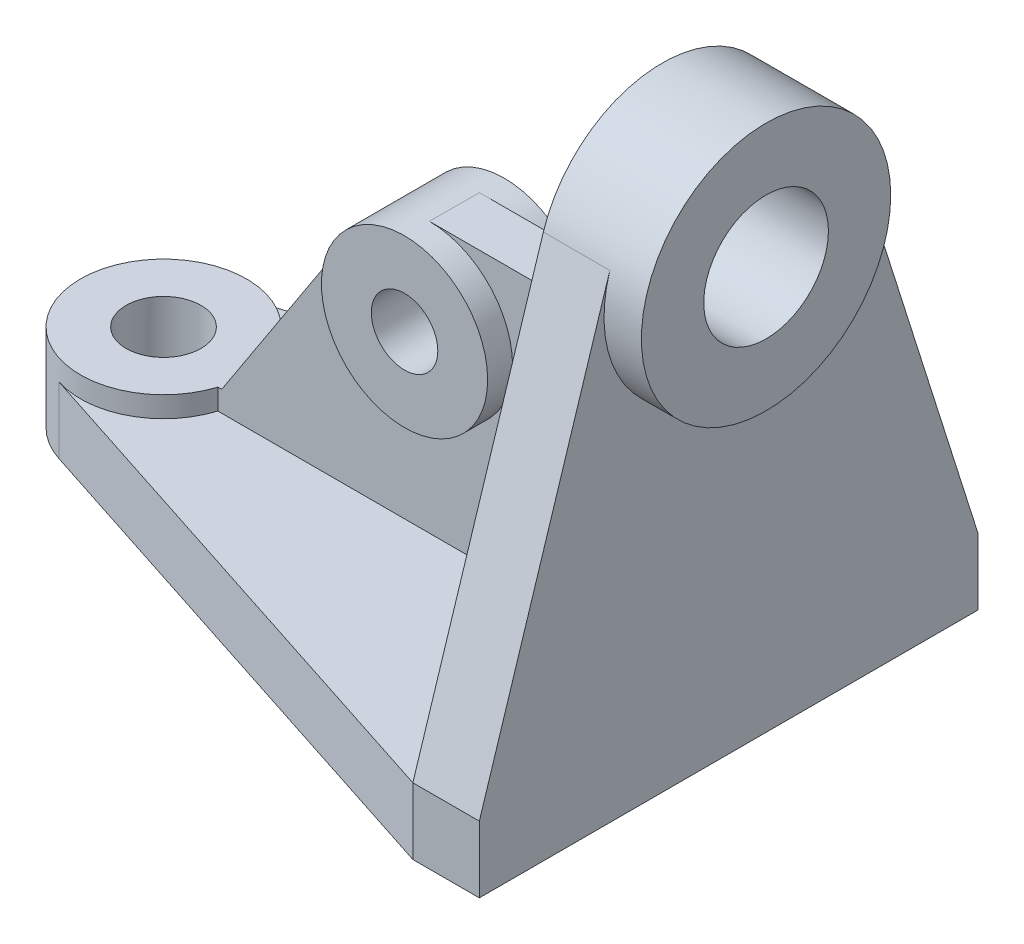
ISO-10303-21;
HEADER;
FILE_DESCRIPTION(('STEP AP214'),'2;1');
FILE_NAME('part.step','',(''),(''),'','','');
FILE_SCHEMA(('AUTOMOTIVE_DESIGN { 1 0 10303 214 1 1 1 1 }'));
ENDSEC;
DATA;
#1=APPLICATION_CONTEXT('core data for automotive mechanical design processes');
#2=APPLICATION_PROTOCOL_DEFINITION('international standard','automotive_design',2000,#1);
#3=PRODUCT_CONTEXT('',#1,'mechanical');
#4=PRODUCT('Part','Part','',(#3));
#5=PRODUCT_RELATED_PRODUCT_CATEGORY('part','',(#4));
#6=PRODUCT_DEFINITION_FORMATION('','',#4);
#7=PRODUCT_DEFINITION_CONTEXT('part definition',#1,'design');
#8=PRODUCT_DEFINITION('design','',#6,#7);
#9=PRODUCT_DEFINITION_SHAPE('','',#8);
#10=(LENGTH_UNIT() NAMED_UNIT(*) SI_UNIT(.MILLI.,.METRE.));
#11=(NAMED_UNIT(*) PLANE_ANGLE_UNIT() SI_UNIT($,.RADIAN.));
#12=(NAMED_UNIT(*) SI_UNIT($,.STERADIAN.) SOLID_ANGLE_UNIT());
#13=UNCERTAINTY_MEASURE_WITH_UNIT(LENGTH_MEASURE(1.E-05),#10,'distance_accuracy_value','');
#14=(GEOMETRIC_REPRESENTATION_CONTEXT(3) GLOBAL_UNCERTAINTY_ASSIGNED_CONTEXT((#13)) GLOBAL_UNIT_ASSIGNED_CONTEXT((#10,
#11,#12)) REPRESENTATION_CONTEXT('',''));
#15=CARTESIAN_POINT('',(0.,0.,0.));
#16=DIRECTION('',(0.,0.,1.));
#17=DIRECTION('',(1.,0.,0.));
#18=AXIS2_PLACEMENT_3D('',#15,#16,#17);
#19=CARTESIAN_POINT('',(-136.,-90.,0.));
#20=DIRECTION('',(0.,-1.,0.));
#21=DIRECTION('',(0.,0.,-1.));
#22=AXIS2_PLACEMENT_3D('',#19,#20,#21);
#23=PLANE('',#22);
#24=CARTESIAN_POINT('',(-136.,-90.,0.));
#25=DIRECTION('',(0.,1.,0.));
#26=DIRECTION('',(0.,0.,1.));
#27=AXIS2_PLACEMENT_3D('',#24,#25,#26);
#28=CIRCLE('',#27,20.);
#29=CARTESIAN_POINT('',(-116.921215971661,-90.,-5.99999999999999));
#30=VERTEX_POINT('',#29);
#31=CARTESIAN_POINT('',(-142.177666107614,-90.,-19.0219988818955));
#32=VERTEX_POINT('',#31);
#33=EDGE_CURVE('E216',#30,#32,#28,.T.);
#34=ORIENTED_EDGE('',*,*,#33,.F.);
#35=DIRECTION('',(1.,0.,0.));
#36=VECTOR('',#35,1.);
#37=CARTESIAN_POINT('',(-16.,-90.,-6.));
#38=LINE('',#37,#36);
#39=CARTESIAN_POINT('',(-16.,-90.,-6.));
#40=VERTEX_POINT('',#39);
#41=EDGE_CURVE('E53',#30,#40,#38,.T.);
#42=ORIENTED_EDGE('',*,*,#41,.T.);
#43=DIRECTION('',(0.,0.,-1.));
#44=VECTOR('',#43,1.);
#45=CARTESIAN_POINT('',(-16.,-90.,60.));
#46=LINE('',#45,#44);
#47=CARTESIAN_POINT('',(-16.,-90.,-60.));
#48=VERTEX_POINT('',#47);
#49=EDGE_CURVE('E276',#40,#48,#46,.T.);
#50=ORIENTED_EDGE('',*,*,#49,.T.);
#51=DIRECTION('',(0.951099944094773,0.,-0.30888330538072));
#52=VECTOR('',#51,1.);
#53=CARTESIAN_POINT('',(-16.,-90.,-60.));
#54=LINE('',#53,#52);
#55=EDGE_CURVE('E230',#32,#48,#54,.T.);
#56=ORIENTED_EDGE('',*,*,#55,.F.);
#57=EDGE_LOOP('',(#34,#42,#50,#56));
#58=FACE_BOUND('',#57,.T.);
#59=ADVANCED_FACE('F39',(#58),#23,.F.);
#60=DIRECTION('',(1.,0.,0.));
#61=VECTOR('',#60,1.);
#62=CARTESIAN_POINT('',(-16.,-90.,6.));
#63=LINE('',#62,#61);
#64=CARTESIAN_POINT('',(-116.921215971661,-90.,5.99999999999999));
#65=VERTEX_POINT('',#64);
#66=CARTESIAN_POINT('',(-16.,-90.,6.));
#67=VERTEX_POINT('',#66);
#68=EDGE_CURVE('E65',#65,#67,#63,.T.);
#69=ORIENTED_EDGE('',*,*,#68,.F.);
#70=CARTESIAN_POINT('',(-142.177666107614,-90.,19.0219988818955));
#71=VERTEX_POINT('',#70);
#72=EDGE_CURVE('E218',#71,#65,#28,.T.);
#73=ORIENTED_EDGE('',*,*,#72,.F.);
#74=DIRECTION('',(-0.951099944094773,0.,-0.30888330538072));
#75=VECTOR('',#74,1.);
#76=CARTESIAN_POINT('',(-142.177666107614,-90.,19.0219988818955));
#77=LINE('',#76,#75);
#78=CARTESIAN_POINT('',(-16.,-90.,60.));
#79=VERTEX_POINT('',#78);
#80=EDGE_CURVE('E224',#79,#71,#77,.T.);
#81=ORIENTED_EDGE('',*,*,#80,.F.);
#82=EDGE_CURVE('E278',#79,#67,#46,.T.);
#83=ORIENTED_EDGE('',*,*,#82,.T.);
#84=EDGE_LOOP('',(#69,#73,#81,#83));
#85=FACE_BOUND('',#84,.T.);
#86=ADVANCED_FACE('F370',(#85),#23,.F.);
#87=CARTESIAN_POINT('',(-16.,-90.,-60.));
#88=DIRECTION('',(0.,0.302169479251962,-0.953254218877943));
#89=DIRECTION('',(0.,0.953254218877943,0.302169479251962));
#90=AXIS2_PLACEMENT_3D('',#87,#88,#89);
#91=PLANE('',#90);
#92=DIRECTION('',(0.,0.953254218877943,0.302169479251962));
#93=VECTOR('',#92,1.);
#94=CARTESIAN_POINT('',(0.,-90.,-60.));
#95=LINE('',#94,#93);
#96=CARTESIAN_POINT('',(0.,-90.,-60.));
#97=VERTEX_POINT('',#96);
#98=CARTESIAN_POINT('',(0.,9.06508437755886,-28.5976265663383));
#99=VERTEX_POINT('',#98);
#100=EDGE_CURVE('E269',#97,#99,#95,.T.);
#101=ORIENTED_EDGE('',*,*,#100,.F.);
#102=DIRECTION('',(1.,0.,0.));
#103=VECTOR('',#102,1.);
#104=CARTESIAN_POINT('',(-16.,-90.,-60.));
#105=LINE('',#104,#103);
#106=EDGE_CURVE('E270',#48,#97,#105,.T.);
#107=ORIENTED_EDGE('',*,*,#106,.F.);
#108=DIRECTION('',(0.,0.953254218877943,0.302169479251962));
#109=VECTOR('',#108,1.);
#110=CARTESIAN_POINT('',(-16.,-90.,-60.));
#111=LINE('',#110,#109);
#112=CARTESIAN_POINT('',(-16.,9.06508437755887,-28.5976265663383));
#113=VERTEX_POINT('',#112);
#114=EDGE_CURVE('E271',#48,#113,#111,.T.);
#115=ORIENTED_EDGE('',*,*,#114,.T.);
#116=DIRECTION('',(1.,0.,0.));
#117=VECTOR('',#116,1.);
#118=CARTESIAN_POINT('',(-16.,9.06508437755887,-28.5976265663383));
#119=LINE('',#118,#117);
#120=EDGE_CURVE('E285',#113,#99,#119,.T.);
#121=ORIENTED_EDGE('',*,*,#120,.T.);
#122=EDGE_LOOP('',(#101,#107,#115,#121));
#123=FACE_BOUND('',#122,.T.);
#124=ADVANCED_FACE('F41',(#123),#91,.T.);
#125=CARTESIAN_POINT('',(-16.,-90.,60.));
#126=DIRECTION('',(0.,0.302169479251962,0.953254218877943));
#127=DIRECTION('',(0.,-0.953254218877943,0.302169479251962));
#128=AXIS2_PLACEMENT_3D('',#125,#126,#127);
#129=PLANE('',#128);
#130=DIRECTION('',(0.,-0.953254218877943,0.302169479251962));
#131=VECTOR('',#130,1.);
#132=CARTESIAN_POINT('',(0.,-90.,60.));
#133=LINE('',#132,#131);
#134=CARTESIAN_POINT('',(0.,9.06508437755887,28.5976265663383));
#135=VERTEX_POINT('',#134);
#136=CARTESIAN_POINT('',(0.,-90.,60.));
#137=VERTEX_POINT('',#136);
#138=EDGE_CURVE('E274',#135,#137,#133,.T.);
#139=ORIENTED_EDGE('',*,*,#138,.F.);
#140=DIRECTION('',(1.,0.,0.));
#141=VECTOR('',#140,1.);
#142=CARTESIAN_POINT('',(-16.,9.06508437755887,28.5976265663383));
#143=LINE('',#142,#141);
#144=CARTESIAN_POINT('',(-16.,9.06508437755887,28.5976265663383));
#145=VERTEX_POINT('',#144);
#146=EDGE_CURVE('E292',#145,#135,#143,.T.);
#147=ORIENTED_EDGE('',*,*,#146,.F.);
#148=DIRECTION('',(0.,-0.953254218877943,0.302169479251962));
#149=VECTOR('',#148,1.);
#150=CARTESIAN_POINT('',(-16.,-90.,60.));
#151=LINE('',#150,#149);
#152=EDGE_CURVE('E280',#145,#79,#151,.T.);
#153=ORIENTED_EDGE('',*,*,#152,.T.);
#154=DIRECTION('',(1.,0.,0.));
#155=VECTOR('',#154,1.);
#156=CARTESIAN_POINT('',(-16.,-90.,60.));
#157=LINE('',#156,#155);
#158=EDGE_CURVE('E289',#79,#137,#157,.T.);
#159=ORIENTED_EDGE('',*,*,#158,.T.);
#160=EDGE_LOOP('',(#139,#147,#153,#159));
#161=FACE_BOUND('',#160,.T.);
#162=ADVANCED_FACE('F310',(#161),#129,.T.);
#163=CARTESIAN_POINT('',(-16.,0.,0.));
#164=DIRECTION('',(1.,0.,0.));
#165=DIRECTION('',(0.,0.,-1.));
#166=AXIS2_PLACEMENT_3D('',#163,#164,#165);
#167=CYLINDRICAL_SURFACE('',#166,30.);
#168=CARTESIAN_POINT('',(0.,0.,0.));
#169=DIRECTION('',(1.,0.,0.));
#170=DIRECTION('',(0.,0.,-1.));
#171=AXIS2_PLACEMENT_3D('',#168,#169,#170);
#172=CIRCLE('',#171,30.);
#173=EDGE_CURVE('E50',#135,#99,#172,.T.);
#174=ORIENTED_EDGE('',*,*,#173,.T.);
#175=ORIENTED_EDGE('',*,*,#120,.F.);
#176=CARTESIAN_POINT('',(-16.,0.,0.));
#177=DIRECTION('',(1.,0.,0.));
#178=DIRECTION('',(0.,0.,-1.));
#179=AXIS2_PLACEMENT_3D('',#176,#177,#178);
#180=CIRCLE('',#179,30.);
#181=EDGE_CURVE('E273',#113,#145,#180,.T.);
#182=ORIENTED_EDGE('',*,*,#181,.T.);
#183=ORIENTED_EDGE('',*,*,#146,.T.);
#184=EDGE_LOOP('',(#174,#175,#182,#183));
#185=FACE_BOUND('',#184,.T.);
#186=CARTESIAN_POINT('',(9.,0.,0.));
#187=DIRECTION('',(1.,0.,0.));
#188=DIRECTION('',(0.,0.,-1.));
#189=AXIS2_PLACEMENT_3D('',#186,#187,#188);
#190=CIRCLE('',#189,30.);
#191=CARTESIAN_POINT('',(9.,0.,-30.));
#192=VERTEX_POINT('',#191);
#193=EDGE_CURVE('E265',#192,#192,#190,.T.);
#194=ORIENTED_EDGE('',*,*,#193,.F.);
#195=EDGE_LOOP('',(#194));
#196=FACE_BOUND('',#195,.T.);
#197=ADVANCED_FACE('F299',(#185,#196),#167,.T.);
#198=CARTESIAN_POINT('',(-16.,0.,0.));
#199=DIRECTION('',(1.,0.,0.));
#200=DIRECTION('',(0.,0.,-1.));
#201=AXIS2_PLACEMENT_3D('',#198,#199,#200);
#202=PLANE('',#201);
#203=CARTESIAN_POINT('',(-16.,0.,0.));
#204=DIRECTION('',(1.,0.,0.));
#205=DIRECTION('',(0.,0.,-1.));
#206=AXIS2_PLACEMENT_3D('',#203,#204,#205);
#207=CIRCLE('',#206,15.);
#208=CARTESIAN_POINT('',(-16.,0.,-15.));
#209=VERTEX_POINT('',#208);
#210=EDGE_CURVE('E264',#209,#209,#207,.T.);
#211=ORIENTED_EDGE('',*,*,#210,.T.);
#212=EDGE_LOOP('',(#211));
#213=FACE_BOUND('',#212,.T.);
#214=ORIENTED_EDGE('',*,*,#152,.F.);
#215=ORIENTED_EDGE('',*,*,#181,.F.);
#216=ORIENTED_EDGE('',*,*,#114,.F.);
#217=ORIENTED_EDGE('',*,*,#49,.F.);
#218=DIRECTION('',(0.,1.,0.));
#219=VECTOR('',#218,1.);
#220=CARTESIAN_POINT('',(-16.,-25.,-6.));
#221=LINE('',#220,#219);
#222=CARTESIAN_POINT('',(-16.,-25.,-6.));
#223=VERTEX_POINT('',#222);
#224=EDGE_CURVE('E202',#40,#223,#221,.T.);
#225=ORIENTED_EDGE('',*,*,#224,.T.);
#226=DIRECTION('',(0.,0.,-1.));
#227=VECTOR('',#226,1.);
#228=CARTESIAN_POINT('',(-16.,-25.,6.));
#229=LINE('',#228,#227);
#230=CARTESIAN_POINT('',(-16.,-25.,6.));
#231=VERTEX_POINT('',#230);
#232=EDGE_CURVE('E209',#231,#223,#229,.T.);
#233=ORIENTED_EDGE('',*,*,#232,.F.);
#234=DIRECTION('',(0.,1.,0.));
#235=VECTOR('',#234,1.);
#236=CARTESIAN_POINT('',(-16.,-25.,6.));
#237=LINE('',#236,#235);
#238=EDGE_CURVE('E197',#67,#231,#237,.T.);
#239=ORIENTED_EDGE('',*,*,#238,.F.);
#240=ORIENTED_EDGE('',*,*,#82,.F.);
#241=EDGE_LOOP('',(#214,#215,#216,#217,#225,#233,#239,#240));
#242=FACE_BOUND('',#241,.T.);
#243=ADVANCED_FACE('F304',(#213,#242),#202,.F.);
#244=CARTESIAN_POINT('',(0.,0.,0.));
#245=DIRECTION('',(1.,0.,0.));
#246=DIRECTION('',(0.,0.,-1.));
#247=AXIS2_PLACEMENT_3D('',#244,#245,#246);
#248=PLANE('',#247);
#249=DIRECTION('',(0.,1.,0.));
#250=VECTOR('',#249,1.);
#251=CARTESIAN_POINT('',(0.,-106.,60.));
#252=LINE('',#251,#250);
#253=CARTESIAN_POINT('',(0.,-106.,60.));
#254=VERTEX_POINT('',#253);
#255=EDGE_CURVE('E258',#254,#137,#252,.T.);
#256=ORIENTED_EDGE('',*,*,#255,.F.);
#257=DIRECTION('',(0.,0.,1.));
#258=VECTOR('',#257,1.);
#259=CARTESIAN_POINT('',(0.,-106.,60.));
#260=LINE('',#259,#258);
#261=CARTESIAN_POINT('',(0.,-106.,-60.));
#262=VERTEX_POINT('',#261);
#263=EDGE_CURVE('E221',#262,#254,#260,.T.);
#264=ORIENTED_EDGE('',*,*,#263,.F.);
#265=DIRECTION('',(0.,1.,0.));
#266=VECTOR('',#265,1.);
#267=CARTESIAN_POINT('',(0.,-106.,-60.));
#268=LINE('',#267,#266);
#269=EDGE_CURVE('E240',#262,#97,#268,.T.);
#270=ORIENTED_EDGE('',*,*,#269,.T.);
#271=ORIENTED_EDGE('',*,*,#100,.T.);
#272=ORIENTED_EDGE('',*,*,#173,.F.);
#273=ORIENTED_EDGE('',*,*,#138,.T.);
#274=EDGE_LOOP('',(#256,#264,#270,#271,#272,#273));
#275=FACE_BOUND('',#274,.T.);
#276=ADVANCED_FACE('F315',(#275),#248,.T.);
#277=CARTESIAN_POINT('',(-16.,0.,0.));
#278=DIRECTION('',(1.,0.,0.));
#279=DIRECTION('',(0.,0.,-1.));
#280=AXIS2_PLACEMENT_3D('',#277,#278,#279);
#281=CYLINDRICAL_SURFACE('',#280,15.);
#282=ORIENTED_EDGE('',*,*,#210,.F.);
#283=EDGE_LOOP('',(#282));
#284=FACE_BOUND('',#283,.T.);
#285=CARTESIAN_POINT('',(9.,0.,0.));
#286=DIRECTION('',(1.,0.,0.));
#287=DIRECTION('',(0.,0.,-1.));
#288=AXIS2_PLACEMENT_3D('',#285,#286,#287);
#289=CIRCLE('',#288,15.);
#290=CARTESIAN_POINT('',(9.,0.,-15.));
#291=VERTEX_POINT('',#290);
#292=EDGE_CURVE('E259',#291,#291,#289,.T.);
#293=ORIENTED_EDGE('',*,*,#292,.T.);
#294=EDGE_LOOP('',(#293));
#295=FACE_BOUND('',#294,.T.);
#296=ADVANCED_FACE('F393',(#284,#295),#281,.F.);
#297=CARTESIAN_POINT('',(9.,0.,0.));
#298=DIRECTION('',(1.,0.,0.));
#299=DIRECTION('',(0.,0.,-1.));
#300=AXIS2_PLACEMENT_3D('',#297,#298,#299);
#301=PLANE('',#300);
#302=ORIENTED_EDGE('',*,*,#292,.F.);
#303=EDGE_LOOP('',(#302));
#304=FACE_BOUND('',#303,.T.);
#305=ORIENTED_EDGE('',*,*,#193,.T.);
#306=EDGE_LOOP('',(#305));
#307=FACE_BOUND('',#306,.T.);
#308=ADVANCED_FACE('F388',(#304,#307),#301,.T.);
#309=CARTESIAN_POINT('',(-136.,-106.,0.));
#310=DIRECTION('',(0.,-1.,0.));
#311=DIRECTION('',(0.,0.,-1.));
#312=AXIS2_PLACEMENT_3D('',#309,#310,#311);
#313=PLANE('',#312);
#314=CARTESIAN_POINT('',(-136.,-106.,0.));
#315=DIRECTION('',(0.,-1.,0.));
#316=DIRECTION('',(0.,0.,-1.));
#317=AXIS2_PLACEMENT_3D('',#314,#315,#316);
#318=CIRCLE('',#317,9.00000000000001);
#319=CARTESIAN_POINT('',(-136.,-106.,-9.00000000000001));
#320=VERTEX_POINT('',#319);
#321=EDGE_CURVE('E217',#320,#320,#318,.T.);
#322=ORIENTED_EDGE('',*,*,#321,.F.);
#323=EDGE_LOOP('',(#322));
#324=FACE_BOUND('',#323,.T.);
#325=ORIENTED_EDGE('',*,*,#263,.T.);
#326=DIRECTION('',(-1.,0.,0.));
#327=VECTOR('',#326,1.);
#328=CARTESIAN_POINT('',(-16.,-106.,60.));
#329=LINE('',#328,#327);
#330=CARTESIAN_POINT('',(-16.,-106.,60.));
#331=VERTEX_POINT('',#330);
#332=EDGE_CURVE('E227',#254,#331,#329,.T.);
#333=ORIENTED_EDGE('',*,*,#332,.T.);
#334=DIRECTION('',(-0.951099944094773,0.,-0.30888330538072));
#335=VECTOR('',#334,1.);
#336=CARTESIAN_POINT('',(-142.177666107614,-106.,19.0219988818955));
#337=LINE('',#336,#335);
#338=CARTESIAN_POINT('',(-142.177666107614,-106.,19.0219988818955));
#339=VERTEX_POINT('',#338);
#340=EDGE_CURVE('E229',#331,#339,#337,.T.);
#341=ORIENTED_EDGE('',*,*,#340,.T.);
#342=CARTESIAN_POINT('',(-136.,-106.,0.));
#343=DIRECTION('',(0.,-1.,0.));
#344=DIRECTION('',(0.,0.,-1.));
#345=AXIS2_PLACEMENT_3D('',#342,#343,#344);
#346=CIRCLE('',#345,20.);
#347=CARTESIAN_POINT('',(-142.177666107614,-106.,-19.0219988818955));
#348=VERTEX_POINT('',#347);
#349=EDGE_CURVE('E232',#339,#348,#346,.T.);
#350=ORIENTED_EDGE('',*,*,#349,.T.);
#351=DIRECTION('',(0.951099944094773,0.,-0.30888330538072));
#352=VECTOR('',#351,1.);
#353=CARTESIAN_POINT('',(-16.,-106.,-60.));
#354=LINE('',#353,#352);
#355=CARTESIAN_POINT('',(-16.,-106.,-60.));
#356=VERTEX_POINT('',#355);
#357=EDGE_CURVE('E233',#348,#356,#354,.T.);
#358=ORIENTED_EDGE('',*,*,#357,.T.);
#359=DIRECTION('',(1.,0.,0.));
#360=VECTOR('',#359,1.);
#361=CARTESIAN_POINT('',(0.,-106.,-60.));
#362=LINE('',#361,#360);
#363=EDGE_CURVE('E231',#356,#262,#362,.T.);
#364=ORIENTED_EDGE('',*,*,#363,.T.);
#365=EDGE_LOOP('',(#325,#333,#341,#350,#358,#364));
#366=FACE_BOUND('',#365,.T.);
#367=ADVANCED_FACE('F319',(#324,#366),#313,.T.);
#368=CARTESIAN_POINT('',(-16.,-106.,60.));
#369=DIRECTION('',(0.,0.,-1.));
#370=DIRECTION('',(-1.,0.,0.));
#371=AXIS2_PLACEMENT_3D('',#368,#369,#370);
#372=PLANE('',#371);
#373=ORIENTED_EDGE('',*,*,#158,.F.);
#374=DIRECTION('',(0.,1.,0.));
#375=VECTOR('',#374,1.);
#376=CARTESIAN_POINT('',(-16.,-106.,60.));
#377=LINE('',#376,#375);
#378=EDGE_CURVE('E251',#331,#79,#377,.T.);
#379=ORIENTED_EDGE('',*,*,#378,.F.);
#380=ORIENTED_EDGE('',*,*,#332,.F.);
#381=ORIENTED_EDGE('',*,*,#255,.T.);
#382=EDGE_LOOP('',(#373,#379,#380,#381));
#383=FACE_BOUND('',#382,.T.);
#384=ADVANCED_FACE('F316',(#383),#372,.F.);
#385=CARTESIAN_POINT('',(-142.177666107614,-106.,19.0219988818955));
#386=DIRECTION('',(0.30888330538072,0.,-0.951099944094773));
#387=DIRECTION('',(-0.951099944094773,0.,-0.30888330538072));
#388=AXIS2_PLACEMENT_3D('',#385,#386,#387);
#389=PLANE('',#388);
#390=ORIENTED_EDGE('',*,*,#80,.T.);
#391=DIRECTION('',(0.,1.,0.));
#392=VECTOR('',#391,1.);
#393=CARTESIAN_POINT('',(-142.177666107614,-106.,19.0219988818955));
#394=LINE('',#393,#392);
#395=EDGE_CURVE('E246',#339,#71,#394,.T.);
#396=ORIENTED_EDGE('',*,*,#395,.F.);
#397=ORIENTED_EDGE('',*,*,#340,.F.);
#398=ORIENTED_EDGE('',*,*,#378,.T.);
#399=EDGE_LOOP('',(#390,#396,#397,#398));
#400=FACE_BOUND('',#399,.T.);
#401=ADVANCED_FACE('F382',(#400),#389,.F.);
#402=CARTESIAN_POINT('',(-136.,-106.,0.));
#403=DIRECTION('',(0.,1.,0.));
#404=DIRECTION('',(0.,0.,1.));
#405=AXIS2_PLACEMENT_3D('',#402,#403,#404);
#406=CYLINDRICAL_SURFACE('',#405,20.);
#407=ORIENTED_EDGE('',*,*,#72,.T.);
#408=DIRECTION('',(0.,1.,0.));
#409=VECTOR('',#408,1.);
#410=CARTESIAN_POINT('',(-116.921215971661,-106.,6.));
#411=LINE('',#410,#409);
#412=CARTESIAN_POINT('',(-116.921215971661,-85.,6.));
#413=VERTEX_POINT('',#412);
#414=EDGE_CURVE('E179',#65,#413,#411,.T.);
#415=ORIENTED_EDGE('',*,*,#414,.T.);
#416=CARTESIAN_POINT('',(-136.,-85.,0.));
#417=DIRECTION('',(0.,1.,0.));
#418=DIRECTION('',(0.,0.,1.));
#419=AXIS2_PLACEMENT_3D('',#416,#417,#418);
#420=CIRCLE('',#419,20.);
#421=CARTESIAN_POINT('',(-116.921215971661,-85.,-6.));
#422=VERTEX_POINT('',#421);
#423=EDGE_CURVE('E172',#422,#413,#420,.T.);
#424=ORIENTED_EDGE('',*,*,#423,.F.);
#425=DIRECTION('',(0.,1.,0.));
#426=VECTOR('',#425,1.);
#427=CARTESIAN_POINT('',(-116.921215971661,-106.,-6.));
#428=LINE('',#427,#426);
#429=EDGE_CURVE('E157',#30,#422,#428,.T.);
#430=ORIENTED_EDGE('',*,*,#429,.F.);
#431=ORIENTED_EDGE('',*,*,#33,.T.);
#432=DIRECTION('',(0.,1.,0.));
#433=VECTOR('',#432,1.);
#434=CARTESIAN_POINT('',(-142.177666107614,-106.,-19.0219988818955));
#435=LINE('',#434,#433);
#436=EDGE_CURVE('E250',#348,#32,#435,.T.);
#437=ORIENTED_EDGE('',*,*,#436,.F.);
#438=ORIENTED_EDGE('',*,*,#349,.F.);
#439=ORIENTED_EDGE('',*,*,#395,.T.);
#440=EDGE_LOOP('',(#407,#415,#424,#430,#431,#437,#438,#439));
#441=FACE_BOUND('',#440,.T.);
#442=ADVANCED_FACE('F379',(#441),#406,.T.);
#443=CARTESIAN_POINT('',(-16.,-106.,-60.));
#444=DIRECTION('',(0.30888330538072,0.,0.951099944094773));
#445=DIRECTION('',(0.951099944094773,0.,-0.30888330538072));
#446=AXIS2_PLACEMENT_3D('',#443,#444,#445);
#447=PLANE('',#446);
#448=ORIENTED_EDGE('',*,*,#55,.T.);
#449=DIRECTION('',(0.,1.,0.));
#450=VECTOR('',#449,1.);
#451=CARTESIAN_POINT('',(-16.,-106.,-60.));
#452=LINE('',#451,#450);
#453=EDGE_CURVE('E244',#356,#48,#452,.T.);
#454=ORIENTED_EDGE('',*,*,#453,.F.);
#455=ORIENTED_EDGE('',*,*,#357,.F.);
#456=ORIENTED_EDGE('',*,*,#436,.T.);
#457=EDGE_LOOP('',(#448,#454,#455,#456));
#458=FACE_BOUND('',#457,.T.);
#459=ADVANCED_FACE('F328',(#458),#447,.F.);
#460=CARTESIAN_POINT('',(0.,-106.,-60.));
#461=DIRECTION('',(0.,0.,1.));
#462=DIRECTION('',(1.,0.,0.));
#463=AXIS2_PLACEMENT_3D('',#460,#461,#462);
#464=PLANE('',#463);
#465=ORIENTED_EDGE('',*,*,#106,.T.);
#466=ORIENTED_EDGE('',*,*,#269,.F.);
#467=ORIENTED_EDGE('',*,*,#363,.F.);
#468=ORIENTED_EDGE('',*,*,#453,.T.);
#469=EDGE_LOOP('',(#465,#466,#467,#468));
#470=FACE_BOUND('',#469,.T.);
#471=ADVANCED_FACE('F324',(#470),#464,.F.);
#472=CARTESIAN_POINT('',(-136.,-106.,0.));
#473=DIRECTION('',(0.,1.,0.));
#474=DIRECTION('',(0.,0.,1.));
#475=AXIS2_PLACEMENT_3D('',#472,#473,#474);
#476=CYLINDRICAL_SURFACE('',#475,9.00000000000001);
#477=CARTESIAN_POINT('',(-136.,-85.,0.));
#478=DIRECTION('',(0.,1.,0.));
#479=DIRECTION('',(0.,0.,1.));
#480=AXIS2_PLACEMENT_3D('',#477,#478,#479);
#481=CIRCLE('',#480,9.00000000000001);
#482=CARTESIAN_POINT('',(-136.,-85.,9.00000000000001));
#483=VERTEX_POINT('',#482);
#484=EDGE_CURVE('E213',#483,#483,#481,.T.);
#485=ORIENTED_EDGE('',*,*,#484,.T.);
#486=EDGE_LOOP('',(#485));
#487=FACE_BOUND('',#486,.T.);
#488=ORIENTED_EDGE('',*,*,#321,.T.);
#489=EDGE_LOOP('',(#488));
#490=FACE_BOUND('',#489,.T.);
#491=ADVANCED_FACE('F380',(#487,#490),#476,.F.);
#492=CARTESIAN_POINT('',(-136.,-85.,0.));
#493=DIRECTION('',(0.,1.,0.));
#494=DIRECTION('',(0.,0.,1.));
#495=AXIS2_PLACEMENT_3D('',#492,#493,#494);
#496=PLANE('',#495);
#497=ORIENTED_EDGE('',*,*,#484,.F.);
#498=EDGE_LOOP('',(#497));
#499=FACE_BOUND('',#498,.T.);
#500=ORIENTED_EDGE('',*,*,#423,.T.);
#501=DIRECTION('',(1.,0.,0.));
#502=VECTOR('',#501,1.);
#503=CARTESIAN_POINT('',(-73.5,-85.,6.));
#504=LINE('',#503,#502);
#505=CARTESIAN_POINT('',(-116.,-85.,6.));
#506=VERTEX_POINT('',#505);
#507=EDGE_CURVE('E164',#506,#413,#504,.F.);
#508=ORIENTED_EDGE('',*,*,#507,.F.);
#509=DIRECTION('',(0.,0.,1.));
#510=VECTOR('',#509,1.);
#511=CARTESIAN_POINT('',(-116.,-85.,0.));
#512=LINE('',#511,#510);
#513=CARTESIAN_POINT('',(-116.,-85.,-6.));
#514=VERTEX_POINT('',#513);
#515=EDGE_CURVE('E149',#514,#506,#512,.T.);
#516=ORIENTED_EDGE('',*,*,#515,.F.);
#517=DIRECTION('',(1.,0.,0.));
#518=VECTOR('',#517,1.);
#519=CARTESIAN_POINT('',(-73.5,-85.,-6.));
#520=LINE('',#519,#518);
#521=EDGE_CURVE('E174',#514,#422,#520,.F.);
#522=ORIENTED_EDGE('',*,*,#521,.T.);
#523=EDGE_LOOP('',(#500,#508,#516,#522));
#524=FACE_BOUND('',#523,.T.);
#525=ADVANCED_FACE('F168',(#499,#524),#496,.T.);
#526=CARTESIAN_POINT('',(-66.,-25.,6.));
#527=DIRECTION('',(0.,-1.,0.));
#528=DIRECTION('',(0.,0.,-1.));
#529=AXIS2_PLACEMENT_3D('',#526,#527,#528);
#530=PLANE('',#529);
#531=DIRECTION('',(-1.,0.,0.));
#532=VECTOR('',#531,1.);
#533=CARTESIAN_POINT('',(-66.,-25.,-6.));
#534=LINE('',#533,#532);
#535=CARTESIAN_POINT('',(-66.,-25.,-6.));
#536=VERTEX_POINT('',#535);
#537=EDGE_CURVE('E191',#223,#536,#534,.T.);
#538=ORIENTED_EDGE('',*,*,#537,.T.);
#539=DIRECTION('',(0.,0.,-1.));
#540=VECTOR('',#539,1.);
#541=CARTESIAN_POINT('',(-66.,-25.,6.));
#542=LINE('',#541,#540);
#543=CARTESIAN_POINT('',(-66.,-25.,6.));
#544=VERTEX_POINT('',#543);
#545=EDGE_CURVE('E205',#544,#536,#542,.T.);
#546=ORIENTED_EDGE('',*,*,#545,.F.);
#547=DIRECTION('',(-1.,0.,0.));
#548=VECTOR('',#547,1.);
#549=CARTESIAN_POINT('',(-66.,-25.,6.));
#550=LINE('',#549,#548);
#551=EDGE_CURVE('E199',#231,#544,#550,.T.);
#552=ORIENTED_EDGE('',*,*,#551,.F.);
#553=ORIENTED_EDGE('',*,*,#232,.T.);
#554=EDGE_LOOP('',(#538,#546,#552,#553));
#555=FACE_BOUND('',#554,.T.);
#556=ADVANCED_FACE('F340',(#555),#530,.F.);
#557=CARTESIAN_POINT('',(-66.,-45.,6.));
#558=DIRECTION('',(0.,0.,1.));
#559=DIRECTION('',(1.,0.,0.));
#560=AXIS2_PLACEMENT_3D('',#557,#558,#559);
#561=PLANE('',#560);
#562=CARTESIAN_POINT('',(-66.,-45.,6.));
#563=DIRECTION('',(0.,0.,-1.));
#564=DIRECTION('',(1.,0.,0.));
#565=AXIS2_PLACEMENT_3D('',#562,#563,#564);
#566=CIRCLE('',#565,20.);
#567=CARTESIAN_POINT('',(-82.7468537176551,-34.0664328529312,6.));
#568=VERTEX_POINT('',#567);
#569=EDGE_CURVE('E170',#544,#568,#566,.T.);
#570=ORIENTED_EDGE('',*,*,#569,.T.);
#571=DIRECTION('',(-0.546678357353441,-0.837342685882753,0.));
#572=VECTOR('',#571,1.);
#573=CARTESIAN_POINT('',(-116.,-85.,6.));
#574=LINE('',#573,#572);
#575=EDGE_CURVE('E155',#568,#506,#574,.T.);
#576=ORIENTED_EDGE('',*,*,#575,.T.);
#577=ORIENTED_EDGE('',*,*,#507,.T.);
#578=ORIENTED_EDGE('',*,*,#414,.F.);
#579=ORIENTED_EDGE('',*,*,#68,.T.);
#580=ORIENTED_EDGE('',*,*,#238,.T.);
#581=ORIENTED_EDGE('',*,*,#551,.T.);
#582=EDGE_LOOP('',(#570,#576,#577,#578,#579,#580,#581));
#583=FACE_BOUND('',#582,.T.);
#584=ADVANCED_FACE('F162',(#583),#561,.T.);
#585=CARTESIAN_POINT('',(-66.,-45.,-6.));
#586=DIRECTION('',(0.,0.,1.));
#587=DIRECTION('',(1.,0.,0.));
#588=AXIS2_PLACEMENT_3D('',#585,#586,#587);
#589=PLANE('',#588);
#590=CARTESIAN_POINT('',(-66.,-45.,-6.));
#591=DIRECTION('',(0.,0.,-1.));
#592=DIRECTION('',(1.,0.,0.));
#593=AXIS2_PLACEMENT_3D('',#590,#591,#592);
#594=CIRCLE('',#593,20.);
#595=CARTESIAN_POINT('',(-82.7468537176551,-34.0664328529312,-6.));
#596=VERTEX_POINT('',#595);
#597=EDGE_CURVE('E192',#536,#596,#594,.T.);
#598=ORIENTED_EDGE('',*,*,#597,.F.);
#599=ORIENTED_EDGE('',*,*,#537,.F.);
#600=ORIENTED_EDGE('',*,*,#224,.F.);
#601=ORIENTED_EDGE('',*,*,#41,.F.);
#602=ORIENTED_EDGE('',*,*,#429,.T.);
#603=ORIENTED_EDGE('',*,*,#521,.F.);
#604=DIRECTION('',(-0.546678357353441,-0.837342685882753,0.));
#605=VECTOR('',#604,1.);
#606=CARTESIAN_POINT('',(-116.,-85.,-6.));
#607=LINE('',#606,#605);
#608=EDGE_CURVE('E152',#596,#514,#607,.T.);
#609=ORIENTED_EDGE('',*,*,#608,.F.);
#610=EDGE_LOOP('',(#598,#599,#600,#601,#602,#603,#609));
#611=FACE_BOUND('',#610,.T.);
#612=ADVANCED_FACE('F336',(#611),#589,.F.);
#613=CARTESIAN_POINT('',(-66.,-45.,12.));
#614=DIRECTION('',(0.,0.,1.));
#615=DIRECTION('',(1.,0.,0.));
#616=AXIS2_PLACEMENT_3D('',#613,#614,#615);
#617=PLANE('',#616);
#618=CARTESIAN_POINT('',(-66.,-45.,12.));
#619=DIRECTION('',(0.,0.,1.));
#620=DIRECTION('',(1.,0.,0.));
#621=AXIS2_PLACEMENT_3D('',#618,#619,#620);
#622=CIRCLE('',#621,20.);
#623=CARTESIAN_POINT('',(-46.,-45.,12.));
#624=VERTEX_POINT('',#623);
#625=EDGE_CURVE('E188',#624,#624,#622,.T.);
#626=ORIENTED_EDGE('',*,*,#625,.T.);
#627=EDGE_LOOP('',(#626));
#628=FACE_BOUND('',#627,.T.);
#629=CARTESIAN_POINT('',(-66.,-45.,12.));
#630=DIRECTION('',(0.,0.,1.));
#631=DIRECTION('',(1.,0.,0.));
#632=AXIS2_PLACEMENT_3D('',#629,#630,#631);
#633=CIRCLE('',#632,8.);
#634=CARTESIAN_POINT('',(-58.,-45.,12.));
#635=VERTEX_POINT('',#634);
#636=EDGE_CURVE('E185',#635,#635,#633,.T.);
#637=ORIENTED_EDGE('',*,*,#636,.F.);
#638=EDGE_LOOP('',(#637));
#639=FACE_BOUND('',#638,.T.);
#640=ADVANCED_FACE('F354',(#628,#639),#617,.T.);
#641=CARTESIAN_POINT('',(-66.,-45.,-12.));
#642=DIRECTION('',(0.,0.,1.));
#643=DIRECTION('',(1.,0.,0.));
#644=AXIS2_PLACEMENT_3D('',#641,#642,#643);
#645=PLANE('',#644);
#646=CARTESIAN_POINT('',(-66.,-45.,-12.));
#647=DIRECTION('',(0.,0.,1.));
#648=DIRECTION('',(1.,0.,0.));
#649=AXIS2_PLACEMENT_3D('',#646,#647,#648);
#650=CIRCLE('',#649,20.);
#651=CARTESIAN_POINT('',(-46.,-45.,-12.));
#652=VERTEX_POINT('',#651);
#653=EDGE_CURVE('E183',#652,#652,#650,.T.);
#654=ORIENTED_EDGE('',*,*,#653,.F.);
#655=EDGE_LOOP('',(#654));
#656=FACE_BOUND('',#655,.T.);
#657=CARTESIAN_POINT('',(-66.,-45.,-12.));
#658=DIRECTION('',(0.,0.,1.));
#659=DIRECTION('',(1.,0.,0.));
#660=AXIS2_PLACEMENT_3D('',#657,#658,#659);
#661=CIRCLE('',#660,8.);
#662=CARTESIAN_POINT('',(-58.,-45.,-12.));
#663=VERTEX_POINT('',#662);
#664=EDGE_CURVE('E182',#663,#663,#661,.T.);
#665=ORIENTED_EDGE('',*,*,#664,.T.);
#666=EDGE_LOOP('',(#665));
#667=FACE_BOUND('',#666,.T.);
#668=ADVANCED_FACE('F347',(#656,#667),#645,.F.);
#669=CARTESIAN_POINT('',(-66.,-45.,12.));
#670=DIRECTION('',(0.,0.,-1.));
#671=DIRECTION('',(-1.,0.,0.));
#672=AXIS2_PLACEMENT_3D('',#669,#670,#671);
#673=CYLINDRICAL_SURFACE('',#672,20.);
#674=ORIENTED_EDGE('',*,*,#569,.F.);
#675=ORIENTED_EDGE('',*,*,#545,.T.);
#676=ORIENTED_EDGE('',*,*,#597,.T.);
#677=DIRECTION('',(0.,0.,-1.));
#678=VECTOR('',#677,1.);
#679=CARTESIAN_POINT('',(-82.7468537176551,-34.0664328529312,12.));
#680=LINE('',#679,#678);
#681=EDGE_CURVE('E11',#568,#596,#680,.T.);
#682=ORIENTED_EDGE('',*,*,#681,.F.);
#683=EDGE_LOOP('',(#674,#675,#676,#682));
#684=FACE_BOUND('',#683,.T.);
#685=ORIENTED_EDGE('',*,*,#625,.F.);
#686=EDGE_LOOP('',(#685));
#687=FACE_BOUND('',#686,.T.);
#688=ORIENTED_EDGE('',*,*,#653,.T.);
#689=EDGE_LOOP('',(#688));
#690=FACE_BOUND('',#689,.T.);
#691=ADVANCED_FACE('F345',(#684,#687,#690),#673,.T.);
#692=CARTESIAN_POINT('',(-66.,-45.,12.));
#693=DIRECTION('',(0.,0.,-1.));
#694=DIRECTION('',(-1.,0.,0.));
#695=AXIS2_PLACEMENT_3D('',#692,#693,#694);
#696=CYLINDRICAL_SURFACE('',#695,8.);
#697=ORIENTED_EDGE('',*,*,#636,.T.);
#698=EDGE_LOOP('',(#697));
#699=FACE_BOUND('',#698,.T.);
#700=ORIENTED_EDGE('',*,*,#664,.F.);
#701=EDGE_LOOP('',(#700));
#702=FACE_BOUND('',#701,.T.);
#703=ADVANCED_FACE('F341',(#699,#702),#696,.F.);
#704=CARTESIAN_POINT('',(-116.,-85.,0.));
#705=DIRECTION('',(-0.837342685882753,0.546678357353441,0.));
#706=DIRECTION('',(-0.546678357353441,-0.837342685882753,0.));
#707=AXIS2_PLACEMENT_3D('',#704,#705,#706);
#708=PLANE('',#707);
#709=ORIENTED_EDGE('',*,*,#575,.F.);
#710=ORIENTED_EDGE('',*,*,#681,.T.);
#711=ORIENTED_EDGE('',*,*,#608,.T.);
#712=ORIENTED_EDGE('',*,*,#515,.T.);
#713=EDGE_LOOP('',(#709,#710,#711,#712));
#714=FACE_BOUND('',#713,.T.);
#715=ADVANCED_FACE('F151',(#714),#708,.T.);
#716=CLOSED_SHELL('',(#59,#86,#124,#162,#197,#243,#276,#296,#308,#367,#384,#401,#442,#459,#471,
#491,#525,#556,#584,#612,#640,#668,#691,#703,#715));
#717=MANIFOLD_SOLID_BREP('B2',#716);
#718=ADVANCED_BREP_SHAPE_REPRESENTATION('',(#18,#717),#14);
#719=SHAPE_DEFINITION_REPRESENTATION(#9,#718);
ENDSEC;
END-ISO-10303-21;
